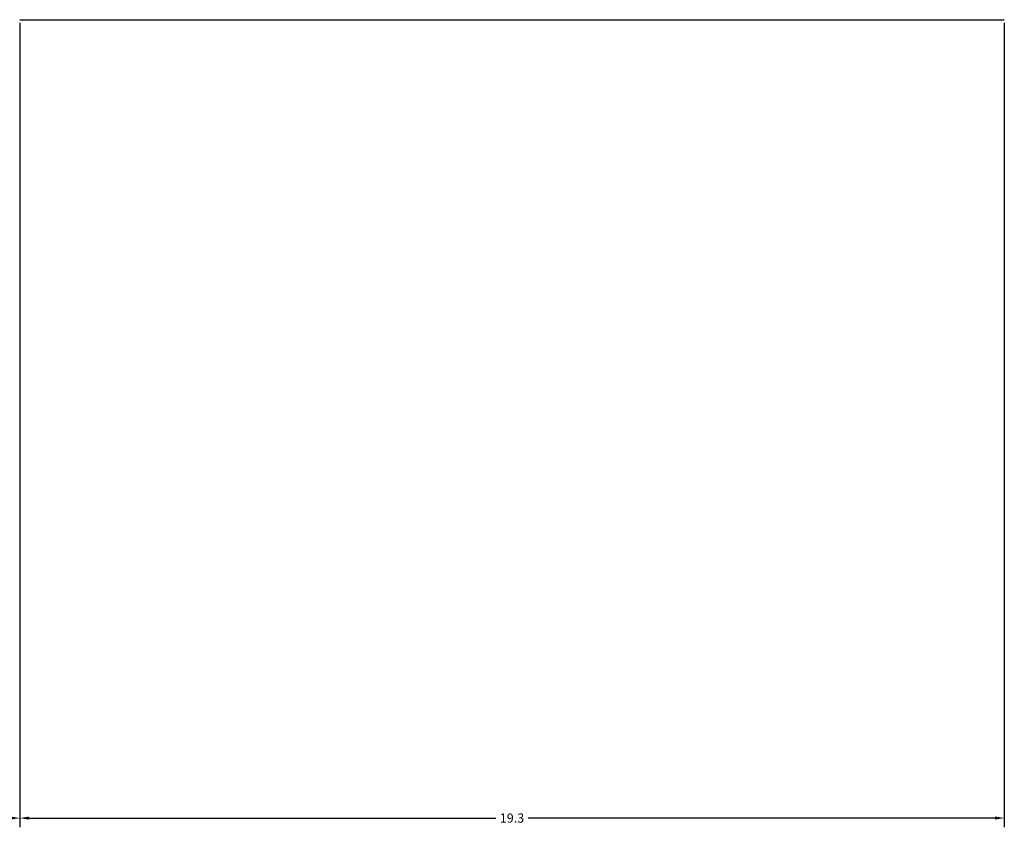
# Model space of a CAD drawing. Units: inches. Extents: x -117 to 121, y -77 to 40.
# Tile 38 of 45: x 90.55 to 109.85, y -77.19 to -61.38. Entities that reach past the tile are written whole.
import ezdxf

# ---------------------------------------------------------------- set-up
doc = ezdxf.new("R2010")
doc.units = ezdxf.units.IN
doc.header["$MEASUREMENT"] = 0
doc.layers.add('A-ANNO-DIMS', color=2, linetype='Continuous', lineweight=18)
doc.layers.add('A-ELEV', color=7, linetype='Continuous', lineweight=25)
doc.styles.get("Standard").update_dxf_attribs({"font": 'arial.ttf'})
doc.dimstyles.get("Standard").update_dxf_attribs({"dimtxt": 0.18, "dimasz": 0.18, "dimexe": 0.18, "dimexo": 0.0625, "dimgap": 0.09, "dimtad": 0, "dimtih": 1, "dimtoh": 1, "dimdec": 4, "dimzin": 0, "dimdsep": 46, "dimtxsty": 'Standard', "dimcen": 0.09, "dimadec": 0, "dimazin": 0, "dimtfac": 1, "dimtdec": 4, "dimtofl": 0, "dimtmove": 0, "dimatfit": 3, "dimfxl": 1, "dimtolj": 1, "dimtzin": 0, "dimarcsym": 0})

# ---------------------------------------------------------------- blocks, each defined once
blk = doc.blocks.new('*D7')
at = {"layer": 'A-ANNO-DIMS', "color": 0, "lineweight": -2, "transparency": 16777216}
for p, q in [((-77.763, -61.431), (-77.763, -77.193)), ((90.549, -61.438), (90.549, -77.193)), ((-77.583, -77.013), (6.008, -77.013)), ((90.369, -77.013), (6.778, -77.013))]:
    blk.add_line(p, q, dxfattribs=at)
at = {"layer": 'A-ANNO-DIMS', "color": 0, "transparency": 16777216}
for points in [[(-77.583, -76.983), (-77.583, -77.043), (-77.763, -77.013)], [(90.369, -76.983), (90.369, -77.043), (90.549, -77.013)]]:
    blk.add_solid(points, dxfattribs=at)
at = {"layer": 'Defpoints', "color": 0, "transparency": 16777216}
for p in [(-77.763, -61.369), (90.549, -61.376), (90.549, -77.013)]:
    blk.add_point(p, dxfattribs=at)
at = {"layer": 'A-ANNO-DIMS', "color": 0, "transparency": 16777216, "insert": (6.393, -77.013), "char_height": 0.18, "attachment_point": 5}
blk.add_mtext('\\A1;168.3', dxfattribs=at)
blk = doc.blocks.new('*D8')
at = {"layer": 'A-ANNO-DIMS', "color": 0, "lineweight": -2, "transparency": 16777216}
for p, q in [((90.549, -61.438), (90.549, -77.193)), ((109.85, -61.438), (109.85, -77.193)), ((90.729, -77.013), (99.884, -77.013)), ((109.67, -77.013), (100.515, -77.013))]:
    blk.add_line(p, q, dxfattribs=at)
at = {"layer": 'A-ANNO-DIMS', "color": 0, "transparency": 16777216}
for points in [[(90.729, -76.983), (90.729, -77.043), (90.549, -77.013)], [(109.67, -76.983), (109.67, -77.043), (109.85, -77.013)]]:
    blk.add_solid(points, dxfattribs=at)
at = {"layer": 'Defpoints', "color": 0, "transparency": 16777216}
for p in [(90.549, -61.376), (109.85, -61.376), (109.85, -77.013)]:
    blk.add_point(p, dxfattribs=at)
at = {"layer": 'A-ANNO-DIMS', "color": 0, "transparency": 16777216, "insert": (100.199, -77.013), "char_height": 0.18, "attachment_point": 5}
blk.add_mtext('\\A1;19.3', dxfattribs=at)
blk = doc.blocks.new('*D31')
at = {"layer": 'A-ANNO-DIMS', "color": 0, "lineweight": -2, "transparency": 16777216}
for p, q in [((87.459, -61.438), (87.459, -77.193)), ((90.549, -61.438), (90.549, -77.193)), ((87.639, -77.013), (88.61, -77.013)), ((90.369, -77.013), (89.397, -77.013))]:
    blk.add_line(p, q, dxfattribs=at)
at = {"layer": 'A-ANNO-DIMS', "color": 0, "transparency": 16777216}
for points in [[(87.639, -76.983), (87.639, -77.043), (87.459, -77.013)], [(90.369, -76.983), (90.369, -77.043), (90.549, -77.013)]]:
    blk.add_solid(points, dxfattribs=at)
at = {"layer": 'Defpoints', "color": 0, "transparency": 16777216}
for p in [(87.459, -61.376), (90.549, -61.376), (90.549, -77.013)]:
    blk.add_point(p, dxfattribs=at)
at = {"layer": 'A-ANNO-DIMS', "color": 0, "transparency": 16777216, "insert": (89.004, -77.013), "char_height": 0.18, "attachment_point": 5}
blk.add_mtext('\\A1;3.090', dxfattribs=at)

msp = doc.modelspace()

# ---------------------------------------------------------------- linework, layer by layer
at = {"layer": 'A-ELEV'}
msp.add_line((90.5486, -61.3756), (109.8502, -61.3756), dxfattribs=at)

# ---------------------------------------------------------------- dimensions: what is measured, and where the dimension line sits
at = {"layer": 'A-ANNO-DIMS'}
for base, p1, p2, override, picture, middle in [((90.5486, -77.0135), (-77.7631, -61.3689), (90.5486, -61.3756), {"dimdec": 1, "dimlfac": 1, "dimrnd": 0, "dimzin": 0, "dimdsep": 46, "dimlunit": 2}, '*D7', (6.3928, -77.0135)), ((90.5486, -77.0135), (87.4587, -61.3756), (90.5486, -61.3756), {"dimdec": 3, "dimlfac": 1, "dimrnd": 0, "dimzin": 0, "dimdsep": 46, "dimlunit": 2}, '*D31', (89.0036, -77.0135)), ((109.8502, -77.0135), (90.5486, -61.3756), (109.8502, -61.3756), {"dimdec": 1, "dimlfac": 1, "dimrnd": 0, "dimzin": 0, "dimdsep": 46, "dimlunit": 2}, '*D8', (100.1994, -77.0135))]:
    dim = msp.add_linear_dim(base=base, p1=p1, p2=p2, dimstyle='Standard', override=override, dxfattribs=at)
    dim.commit()
    dim.dimension.update_dxf_attribs({"geometry": picture, "text_midpoint": middle})

doc.saveas('drawing.dxf')
